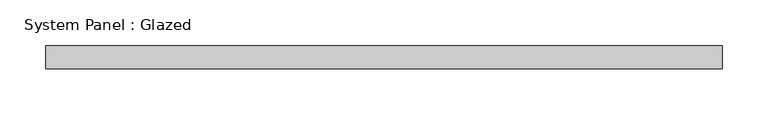
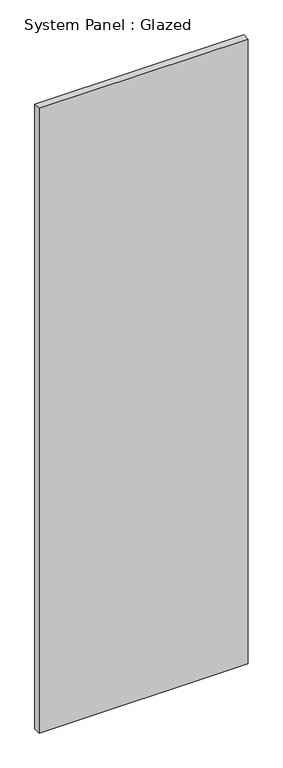
"""IFC4 building model written with IfcOpenShell, lengths in millimetres: plate geometry, System Panel : Glazed."""

from ifc_helpers import new_model, si_unit, origin, origin_with_axes, place, context, project, spatial, polyline, outline, extrude, source, transform, mapped, element, save


def system_panel_glazed_65d20654(model_context):
    return source(origin(), model_context, "Body", "SweptSolid", [
        extrude(outline(polyline([(371.475, 19.05), (-371.475, 19.05), (-371.475, 44.45), (371.475, 44.45), (371.475, 19.05)])), origin_with_axes(), (0.0, 0.0, 1.0), 2343.15),
    ])


if __name__ == "__main__":
    model = new_model("IFC4")
    model_context = context("Model", 3, world=origin())
    ifc_project = project(units=[si_unit("LENGTHUNIT", "METRE", prefix="MILLI")], contexts=[model_context])
    site = spatial("IfcSite", under=ifc_project)
    building = spatial("IfcBuilding", under=site)
    placement = place(None, origin())
    system_panel_glazed_shape = system_panel_glazed_65d20654(model_context)
    element("IfcPlate", 1, ObjectType="System Panel : Glazed", at=placement, inside=building, context=model_context, shape_type="MappedRepresentation", body=[
        mapped(system_panel_glazed_shape, transform((0.0, 0.0, 0.0), x_axis=(1.0, 0.0, 0.0), y_axis=(0.0, 1.0, 0.0), z_axis=(0.0, 0.0, 1.0))),
    ])
    save(model, "model.ifc")

# Revit data of these elements
# Type "System Panel : Glazed"
#   Construction Type Id = "GSP4R"
#   Analytic Construction = "1/8 in Pilkington single glazing"
#   Visual Light Transmittance = 0.9
#   Solar Heat Gain Coefficient = 0.86
#   Heat Transfer Coefficient (U) = 1.18115 BTU/(h·ft²·°F)
#   Define Thermal Properties by = 1
# Element 1 (IfcPlate, "System Panel : Glazed")
#   Materials on its faces: "Glass"
# Materials
#   "Glass": class "Glass", colour RGB 0 128 192, transparency 0.75, Description = "Soda Lime Glass", Cost = 0
